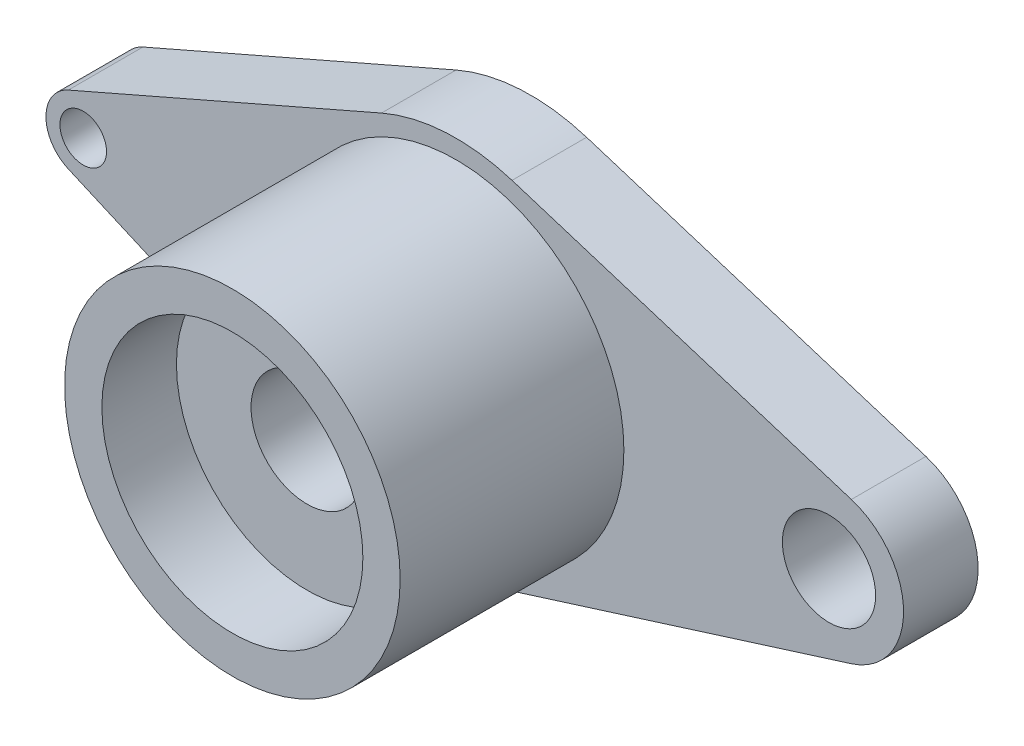
ISO-10303-21;
HEADER;
FILE_DESCRIPTION(('STEP AP214'),'2;1');
FILE_NAME('part.step','',(''),(''),'','','');
FILE_SCHEMA(('AUTOMOTIVE_DESIGN { 1 0 10303 214 1 1 1 1 }'));
ENDSEC;
DATA;
#1=APPLICATION_CONTEXT('core data for automotive mechanical design processes');
#2=APPLICATION_PROTOCOL_DEFINITION('international standard','automotive_design',2000,#1);
#3=PRODUCT_CONTEXT('',#1,'mechanical');
#4=PRODUCT('Part','Part','',(#3));
#5=PRODUCT_RELATED_PRODUCT_CATEGORY('part','',(#4));
#6=PRODUCT_DEFINITION_FORMATION('','',#4);
#7=PRODUCT_DEFINITION_CONTEXT('part definition',#1,'design');
#8=PRODUCT_DEFINITION('design','',#6,#7);
#9=PRODUCT_DEFINITION_SHAPE('','',#8);
#10=(LENGTH_UNIT() NAMED_UNIT(*) SI_UNIT(.MILLI.,.METRE.));
#11=(NAMED_UNIT(*) PLANE_ANGLE_UNIT() SI_UNIT($,.RADIAN.));
#12=(NAMED_UNIT(*) SI_UNIT($,.STERADIAN.) SOLID_ANGLE_UNIT());
#13=UNCERTAINTY_MEASURE_WITH_UNIT(LENGTH_MEASURE(1.E-05),#10,'distance_accuracy_value','');
#14=(GEOMETRIC_REPRESENTATION_CONTEXT(3) GLOBAL_UNCERTAINTY_ASSIGNED_CONTEXT((#13)) GLOBAL_UNIT_ASSIGNED_CONTEXT((#10,
#11,#12)) REPRESENTATION_CONTEXT('',''));
#15=CARTESIAN_POINT('',(0.,0.,0.));
#16=DIRECTION('',(0.,0.,1.));
#17=DIRECTION('',(1.,0.,0.));
#18=AXIS2_PLACEMENT_3D('',#15,#16,#17);
#19=CARTESIAN_POINT('',(0.,0.,20.));
#20=DIRECTION('',(0.,0.,1.));
#21=DIRECTION('',(1.,0.,0.));
#22=AXIS2_PLACEMENT_3D('',#19,#20,#21);
#23=PLANE('',#22);
#24=CARTESIAN_POINT('',(100.,0.,20.));
#25=DIRECTION('',(0.,0.,1.));
#26=DIRECTION('',(1.,0.,0.));
#27=AXIS2_PLACEMENT_3D('',#24,#25,#26);
#28=CIRCLE('',#27,45.);
#29=CARTESIAN_POINT('',(145.,0.,20.));
#30=VERTEX_POINT('',#29);
#31=EDGE_CURVE('E200',#30,#30,#28,.T.);
#32=ORIENTED_EDGE('',*,*,#31,.F.);
#33=EDGE_LOOP('',(#32));
#34=FACE_BOUND('',#33,.T.);
#35=CARTESIAN_POINT('',(0.,0.,20.));
#36=DIRECTION('',(0.,0.,1.));
#37=DIRECTION('',(1.,0.,0.));
#38=AXIS2_PLACEMENT_3D('',#35,#36,#37);
#39=CIRCLE('',#38,6.25);
#40=CARTESIAN_POINT('',(6.25,0.,20.));
#41=VERTEX_POINT('',#40);
#42=EDGE_CURVE('E150',#41,#41,#39,.T.);
#43=ORIENTED_EDGE('',*,*,#42,.F.);
#44=EDGE_LOOP('',(#43));
#45=FACE_BOUND('',#44,.T.);
#46=CARTESIAN_POINT('',(0.,0.,20.));
#47=DIRECTION('',(0.,0.,1.));
#48=DIRECTION('',(1.,0.,0.));
#49=AXIS2_PLACEMENT_3D('',#46,#47,#48);
#50=CIRCLE('',#49,10.);
#51=CARTESIAN_POINT('',(-4.,9.16515138991168,20.));
#52=VERTEX_POINT('',#51);
#53=CARTESIAN_POINT('',(-4.,-9.16515138991168,20.));
#54=VERTEX_POINT('',#53);
#55=EDGE_CURVE('E158',#52,#54,#50,.T.);
#56=ORIENTED_EDGE('',*,*,#55,.T.);
#57=DIRECTION('',(0.916515138991168,-0.4,0.));
#58=VECTOR('',#57,1.);
#59=CARTESIAN_POINT('',(-4.,-9.16515138991168,20.));
#60=LINE('',#59,#58);
#61=CARTESIAN_POINT('',(80.,-45.8257569495584,20.));
#62=VERTEX_POINT('',#61);
#63=EDGE_CURVE('E106',#54,#62,#60,.T.);
#64=ORIENTED_EDGE('',*,*,#63,.T.);
#65=CARTESIAN_POINT('',(100.,0.,20.));
#66=DIRECTION('',(0.,0.,1.));
#67=DIRECTION('',(1.,0.,0.));
#68=AXIS2_PLACEMENT_3D('',#65,#66,#67);
#69=CIRCLE('',#68,50.);
#70=CARTESIAN_POINT('',(115.,-47.6969600708473,20.));
#71=VERTEX_POINT('',#70);
#72=EDGE_CURVE('E212',#62,#71,#69,.T.);
#73=ORIENTED_EDGE('',*,*,#72,.T.);
#74=DIRECTION('',(0.953939201416946,0.3,0.));
#75=VECTOR('',#74,1.);
#76=CARTESIAN_POINT('',(115.,-47.6969600708473,20.));
#77=LINE('',#76,#75);
#78=CARTESIAN_POINT('',(206.,-19.0787840283389,20.));
#79=VERTEX_POINT('',#78);
#80=EDGE_CURVE('E216',#71,#79,#77,.T.);
#81=ORIENTED_EDGE('',*,*,#80,.T.);
#82=CARTESIAN_POINT('',(200.,0.,20.));
#83=DIRECTION('',(0.,0.,1.));
#84=DIRECTION('',(1.,0.,0.));
#85=AXIS2_PLACEMENT_3D('',#82,#83,#84);
#86=CIRCLE('',#85,20.);
#87=CARTESIAN_POINT('',(206.,19.0787840283389,20.));
#88=VERTEX_POINT('',#87);
#89=EDGE_CURVE('E123',#79,#88,#86,.T.);
#90=ORIENTED_EDGE('',*,*,#89,.T.);
#91=DIRECTION('',(-0.953939201416946,0.3,0.));
#92=VECTOR('',#91,1.);
#93=CARTESIAN_POINT('',(115.,47.6969600708473,20.));
#94=LINE('',#93,#92);
#95=CARTESIAN_POINT('',(115.,47.6969600708473,20.));
#96=VERTEX_POINT('',#95);
#97=EDGE_CURVE('E118',#88,#96,#94,.T.);
#98=ORIENTED_EDGE('',*,*,#97,.T.);
#99=CARTESIAN_POINT('',(100.,0.,20.));
#100=DIRECTION('',(0.,0.,1.));
#101=DIRECTION('',(1.,0.,0.));
#102=AXIS2_PLACEMENT_3D('',#99,#100,#101);
#103=CIRCLE('',#102,50.);
#104=CARTESIAN_POINT('',(80.,45.8257569495584,20.));
#105=VERTEX_POINT('',#104);
#106=EDGE_CURVE('E125',#96,#105,#103,.T.);
#107=ORIENTED_EDGE('',*,*,#106,.T.);
#108=DIRECTION('',(-0.916515138991168,-0.4,0.));
#109=VECTOR('',#108,1.);
#110=CARTESIAN_POINT('',(-4.,9.16515138991168,20.));
#111=LINE('',#110,#109);
#112=EDGE_CURVE('E61',#105,#52,#111,.T.);
#113=ORIENTED_EDGE('',*,*,#112,.T.);
#114=EDGE_LOOP('',(#56,#64,#73,#81,#90,#98,#107,#113));
#115=FACE_BOUND('',#114,.T.);
#116=CARTESIAN_POINT('',(200.,0.,20.));
#117=DIRECTION('',(0.,0.,1.));
#118=DIRECTION('',(1.,0.,0.));
#119=AXIS2_PLACEMENT_3D('',#116,#117,#118);
#120=CIRCLE('',#119,12.5);
#121=CARTESIAN_POINT('',(212.5,0.,20.));
#122=VERTEX_POINT('',#121);
#123=EDGE_CURVE('E206',#122,#122,#120,.T.);
#124=ORIENTED_EDGE('',*,*,#123,.F.);
#125=EDGE_LOOP('',(#124));
#126=FACE_BOUND('',#125,.T.);
#127=ADVANCED_FACE('F44',(#34,#45,#115,#126),#23,.T.);
#128=CARTESIAN_POINT('',(0.,0.,0.));
#129=DIRECTION('',(0.,0.,1.));
#130=DIRECTION('',(1.,0.,0.));
#131=AXIS2_PLACEMENT_3D('',#128,#129,#130);
#132=PLANE('',#131);
#133=CARTESIAN_POINT('',(0.,0.,0.));
#134=DIRECTION('',(0.,0.,1.));
#135=DIRECTION('',(1.,0.,0.));
#136=AXIS2_PLACEMENT_3D('',#133,#134,#135);
#137=CIRCLE('',#136,10.);
#138=CARTESIAN_POINT('',(-4.,9.16515138991168,0.));
#139=VERTEX_POINT('',#138);
#140=CARTESIAN_POINT('',(-4.,-9.16515138991168,0.));
#141=VERTEX_POINT('',#140);
#142=EDGE_CURVE('E141',#139,#141,#137,.T.);
#143=ORIENTED_EDGE('',*,*,#142,.F.);
#144=DIRECTION('',(-0.916515138991168,-0.4,0.));
#145=VECTOR('',#144,1.);
#146=CARTESIAN_POINT('',(-4.,9.16515138991168,0.));
#147=LINE('',#146,#145);
#148=CARTESIAN_POINT('',(80.,45.8257569495584,0.));
#149=VERTEX_POINT('',#148);
#150=EDGE_CURVE('E100',#149,#139,#147,.T.);
#151=ORIENTED_EDGE('',*,*,#150,.F.);
#152=CARTESIAN_POINT('',(100.,0.,0.));
#153=DIRECTION('',(0.,0.,1.));
#154=DIRECTION('',(1.,0.,0.));
#155=AXIS2_PLACEMENT_3D('',#152,#153,#154);
#156=CIRCLE('',#155,50.);
#157=CARTESIAN_POINT('',(115.,47.6969600708473,0.));
#158=VERTEX_POINT('',#157);
#159=EDGE_CURVE('E93',#158,#149,#156,.T.);
#160=ORIENTED_EDGE('',*,*,#159,.F.);
#161=DIRECTION('',(-0.953939201416946,0.3,0.));
#162=VECTOR('',#161,1.);
#163=CARTESIAN_POINT('',(115.,47.6969600708473,0.));
#164=LINE('',#163,#162);
#165=CARTESIAN_POINT('',(206.,19.0787840283389,0.));
#166=VERTEX_POINT('',#165);
#167=EDGE_CURVE('E135',#166,#158,#164,.T.);
#168=ORIENTED_EDGE('',*,*,#167,.F.);
#169=CARTESIAN_POINT('',(200.,0.,0.));
#170=DIRECTION('',(0.,0.,1.));
#171=DIRECTION('',(1.,0.,0.));
#172=AXIS2_PLACEMENT_3D('',#169,#170,#171);
#173=CIRCLE('',#172,20.);
#174=CARTESIAN_POINT('',(206.,-19.0787840283389,0.));
#175=VERTEX_POINT('',#174);
#176=EDGE_CURVE('E153',#175,#166,#173,.T.);
#177=ORIENTED_EDGE('',*,*,#176,.F.);
#178=DIRECTION('',(0.953939201416946,0.3,0.));
#179=VECTOR('',#178,1.);
#180=CARTESIAN_POINT('',(115.,-47.6969600708473,0.));
#181=LINE('',#180,#179);
#182=CARTESIAN_POINT('',(115.,-47.6969600708473,0.));
#183=VERTEX_POINT('',#182);
#184=EDGE_CURVE('E151',#183,#175,#181,.T.);
#185=ORIENTED_EDGE('',*,*,#184,.F.);
#186=CARTESIAN_POINT('',(100.,0.,0.));
#187=DIRECTION('',(0.,0.,1.));
#188=DIRECTION('',(1.,0.,0.));
#189=AXIS2_PLACEMENT_3D('',#186,#187,#188);
#190=CIRCLE('',#189,50.);
#191=CARTESIAN_POINT('',(80.,-45.8257569495584,0.));
#192=VERTEX_POINT('',#191);
#193=EDGE_CURVE('E149',#192,#183,#190,.T.);
#194=ORIENTED_EDGE('',*,*,#193,.F.);
#195=DIRECTION('',(0.916515138991168,-0.4,0.));
#196=VECTOR('',#195,1.);
#197=CARTESIAN_POINT('',(-4.,-9.16515138991168,0.));
#198=LINE('',#197,#196);
#199=EDGE_CURVE('E148',#141,#192,#198,.T.);
#200=ORIENTED_EDGE('',*,*,#199,.F.);
#201=EDGE_LOOP('',(#143,#151,#160,#168,#177,#185,#194,#200));
#202=FACE_BOUND('',#201,.T.);
#203=CARTESIAN_POINT('',(0.,0.,0.));
#204=DIRECTION('',(0.,0.,1.));
#205=DIRECTION('',(1.,0.,0.));
#206=AXIS2_PLACEMENT_3D('',#203,#204,#205);
#207=CIRCLE('',#206,6.25);
#208=CARTESIAN_POINT('',(6.25,0.,0.));
#209=VERTEX_POINT('',#208);
#210=EDGE_CURVE('E201',#209,#209,#207,.T.);
#211=ORIENTED_EDGE('',*,*,#210,.T.);
#212=EDGE_LOOP('',(#211));
#213=FACE_BOUND('',#212,.T.);
#214=CARTESIAN_POINT('',(200.,0.,0.));
#215=DIRECTION('',(0.,0.,1.));
#216=DIRECTION('',(1.,0.,0.));
#217=AXIS2_PLACEMENT_3D('',#214,#215,#216);
#218=CIRCLE('',#217,12.5);
#219=CARTESIAN_POINT('',(212.5,0.,0.));
#220=VERTEX_POINT('',#219);
#221=EDGE_CURVE('E207',#220,#220,#218,.T.);
#222=ORIENTED_EDGE('',*,*,#221,.T.);
#223=EDGE_LOOP('',(#222));
#224=FACE_BOUND('',#223,.T.);
#225=ADVANCED_FACE('F188',(#202,#213,#224),#132,.F.);
#226=CARTESIAN_POINT('',(0.,0.,20.));
#227=DIRECTION('',(0.,0.,-1.));
#228=DIRECTION('',(-1.,0.,0.));
#229=AXIS2_PLACEMENT_3D('',#226,#227,#228);
#230=CYLINDRICAL_SURFACE('',#229,10.);
#231=ORIENTED_EDGE('',*,*,#142,.T.);
#232=DIRECTION('',(0.,0.,-1.));
#233=VECTOR('',#232,1.);
#234=CARTESIAN_POINT('',(-4.,-9.16515138991168,20.));
#235=LINE('',#234,#233);
#236=EDGE_CURVE('E174',#54,#141,#235,.T.);
#237=ORIENTED_EDGE('',*,*,#236,.F.);
#238=ORIENTED_EDGE('',*,*,#55,.F.);
#239=DIRECTION('',(0.,0.,-1.));
#240=VECTOR('',#239,1.);
#241=CARTESIAN_POINT('',(-4.,9.16515138991168,20.));
#242=LINE('',#241,#240);
#243=EDGE_CURVE('E136',#52,#139,#242,.T.);
#244=ORIENTED_EDGE('',*,*,#243,.T.);
#245=EDGE_LOOP('',(#231,#237,#238,#244));
#246=FACE_BOUND('',#245,.T.);
#247=ADVANCED_FACE('F50',(#246),#230,.T.);
#248=CARTESIAN_POINT('',(-4.,-9.16515138991168,20.));
#249=DIRECTION('',(0.4,0.916515138991168,0.));
#250=DIRECTION('',(-0.916515138991168,0.4,0.));
#251=AXIS2_PLACEMENT_3D('',#248,#249,#250);
#252=PLANE('',#251);
#253=ORIENTED_EDGE('',*,*,#199,.T.);
#254=DIRECTION('',(0.,0.,-1.));
#255=VECTOR('',#254,1.);
#256=CARTESIAN_POINT('',(80.,-45.8257569495584,20.));
#257=LINE('',#256,#255);
#258=EDGE_CURVE('E169',#62,#192,#257,.T.);
#259=ORIENTED_EDGE('',*,*,#258,.F.);
#260=ORIENTED_EDGE('',*,*,#63,.F.);
#261=ORIENTED_EDGE('',*,*,#236,.T.);
#262=EDGE_LOOP('',(#253,#259,#260,#261));
#263=FACE_BOUND('',#262,.T.);
#264=ADVANCED_FACE('F251',(#263),#252,.F.);
#265=CARTESIAN_POINT('',(100.,0.,20.));
#266=DIRECTION('',(0.,0.,-1.));
#267=DIRECTION('',(-1.,0.,0.));
#268=AXIS2_PLACEMENT_3D('',#265,#266,#267);
#269=CYLINDRICAL_SURFACE('',#268,50.);
#270=ORIENTED_EDGE('',*,*,#193,.T.);
#271=DIRECTION('',(0.,0.,-1.));
#272=VECTOR('',#271,1.);
#273=CARTESIAN_POINT('',(115.,-47.6969600708473,20.));
#274=LINE('',#273,#272);
#275=EDGE_CURVE('E164',#71,#183,#274,.T.);
#276=ORIENTED_EDGE('',*,*,#275,.F.);
#277=ORIENTED_EDGE('',*,*,#72,.F.);
#278=ORIENTED_EDGE('',*,*,#258,.T.);
#279=EDGE_LOOP('',(#270,#276,#277,#278));
#280=FACE_BOUND('',#279,.T.);
#281=ADVANCED_FACE('F253',(#280),#269,.T.);
#282=CARTESIAN_POINT('',(115.,-47.6969600708473,20.));
#283=DIRECTION('',(-0.3,0.953939201416946,0.));
#284=DIRECTION('',(-0.953939201416946,-0.3,0.));
#285=AXIS2_PLACEMENT_3D('',#282,#283,#284);
#286=PLANE('',#285);
#287=ORIENTED_EDGE('',*,*,#184,.T.);
#288=DIRECTION('',(0.,0.,-1.));
#289=VECTOR('',#288,1.);
#290=CARTESIAN_POINT('',(206.,-19.0787840283389,20.));
#291=LINE('',#290,#289);
#292=EDGE_CURVE('E165',#79,#175,#291,.T.);
#293=ORIENTED_EDGE('',*,*,#292,.F.);
#294=ORIENTED_EDGE('',*,*,#80,.F.);
#295=ORIENTED_EDGE('',*,*,#275,.T.);
#296=EDGE_LOOP('',(#287,#293,#294,#295));
#297=FACE_BOUND('',#296,.T.);
#298=ADVANCED_FACE('F225',(#297),#286,.F.);
#299=CARTESIAN_POINT('',(200.,0.,20.));
#300=DIRECTION('',(0.,0.,-1.));
#301=DIRECTION('',(-1.,0.,0.));
#302=AXIS2_PLACEMENT_3D('',#299,#300,#301);
#303=CYLINDRICAL_SURFACE('',#302,20.);
#304=ORIENTED_EDGE('',*,*,#176,.T.);
#305=DIRECTION('',(0.,0.,-1.));
#306=VECTOR('',#305,1.);
#307=CARTESIAN_POINT('',(206.,19.0787840283389,20.));
#308=LINE('',#307,#306);
#309=EDGE_CURVE('E133',#88,#166,#308,.T.);
#310=ORIENTED_EDGE('',*,*,#309,.F.);
#311=ORIENTED_EDGE('',*,*,#89,.F.);
#312=ORIENTED_EDGE('',*,*,#292,.T.);
#313=EDGE_LOOP('',(#304,#310,#311,#312));
#314=FACE_BOUND('',#313,.T.);
#315=ADVANCED_FACE('F229',(#314),#303,.T.);
#316=CARTESIAN_POINT('',(115.,47.6969600708473,20.));
#317=DIRECTION('',(-0.3,-0.953939201416946,0.));
#318=DIRECTION('',(0.953939201416946,-0.3,0.));
#319=AXIS2_PLACEMENT_3D('',#316,#317,#318);
#320=PLANE('',#319);
#321=ORIENTED_EDGE('',*,*,#167,.T.);
#322=DIRECTION('',(0.,0.,-1.));
#323=VECTOR('',#322,1.);
#324=CARTESIAN_POINT('',(115.,47.6969600708473,20.));
#325=LINE('',#324,#323);
#326=EDGE_CURVE('E128',#96,#158,#325,.T.);
#327=ORIENTED_EDGE('',*,*,#326,.F.);
#328=ORIENTED_EDGE('',*,*,#97,.F.);
#329=ORIENTED_EDGE('',*,*,#309,.T.);
#330=EDGE_LOOP('',(#321,#327,#328,#329));
#331=FACE_BOUND('',#330,.T.);
#332=ADVANCED_FACE('F134',(#331),#320,.F.);
#333=CARTESIAN_POINT('',(100.,0.,20.));
#334=DIRECTION('',(0.,0.,-1.));
#335=DIRECTION('',(-1.,0.,0.));
#336=AXIS2_PLACEMENT_3D('',#333,#334,#335);
#337=CYLINDRICAL_SURFACE('',#336,50.);
#338=ORIENTED_EDGE('',*,*,#159,.T.);
#339=DIRECTION('',(0.,0.,-1.));
#340=VECTOR('',#339,1.);
#341=CARTESIAN_POINT('',(80.,45.8257569495584,20.));
#342=LINE('',#341,#340);
#343=EDGE_CURVE('E132',#105,#149,#342,.T.);
#344=ORIENTED_EDGE('',*,*,#343,.F.);
#345=ORIENTED_EDGE('',*,*,#106,.F.);
#346=ORIENTED_EDGE('',*,*,#326,.T.);
#347=EDGE_LOOP('',(#338,#344,#345,#346));
#348=FACE_BOUND('',#347,.T.);
#349=ADVANCED_FACE('F139',(#348),#337,.T.);
#350=CARTESIAN_POINT('',(-4.,9.16515138991168,20.));
#351=DIRECTION('',(0.4,-0.916515138991168,0.));
#352=DIRECTION('',(0.916515138991168,0.4,0.));
#353=AXIS2_PLACEMENT_3D('',#350,#351,#352);
#354=PLANE('',#353);
#355=ORIENTED_EDGE('',*,*,#150,.T.);
#356=ORIENTED_EDGE('',*,*,#243,.F.);
#357=ORIENTED_EDGE('',*,*,#112,.F.);
#358=ORIENTED_EDGE('',*,*,#343,.T.);
#359=EDGE_LOOP('',(#355,#356,#357,#358));
#360=FACE_BOUND('',#359,.T.);
#361=ADVANCED_FACE('F235',(#360),#354,.F.);
#362=CARTESIAN_POINT('',(0.,0.,20.));
#363=DIRECTION('',(0.,0.,-1.));
#364=DIRECTION('',(-1.,0.,0.));
#365=AXIS2_PLACEMENT_3D('',#362,#363,#364);
#366=CYLINDRICAL_SURFACE('',#365,6.25);
#367=ORIENTED_EDGE('',*,*,#42,.T.);
#368=EDGE_LOOP('',(#367));
#369=FACE_BOUND('',#368,.T.);
#370=ORIENTED_EDGE('',*,*,#210,.F.);
#371=EDGE_LOOP('',(#370));
#372=FACE_BOUND('',#371,.T.);
#373=ADVANCED_FACE('F233',(#369,#372),#366,.F.);
#374=CARTESIAN_POINT('',(200.,0.,20.));
#375=DIRECTION('',(0.,0.,-1.));
#376=DIRECTION('',(-1.,0.,0.));
#377=AXIS2_PLACEMENT_3D('',#374,#375,#376);
#378=CYLINDRICAL_SURFACE('',#377,12.5);
#379=ORIENTED_EDGE('',*,*,#123,.T.);
#380=EDGE_LOOP('',(#379));
#381=FACE_BOUND('',#380,.T.);
#382=ORIENTED_EDGE('',*,*,#221,.F.);
#383=EDGE_LOOP('',(#382));
#384=FACE_BOUND('',#383,.T.);
#385=ADVANCED_FACE('F241',(#381,#384),#378,.F.);
#386=CARTESIAN_POINT('',(100.,0.,80.));
#387=DIRECTION('',(0.,0.,1.));
#388=DIRECTION('',(1.,0.,0.));
#389=AXIS2_PLACEMENT_3D('',#386,#387,#388);
#390=PLANE('',#389);
#391=CARTESIAN_POINT('',(100.,0.,80.));
#392=DIRECTION('',(0.,0.,1.));
#393=DIRECTION('',(1.,0.,0.));
#394=AXIS2_PLACEMENT_3D('',#391,#392,#393);
#395=CIRCLE('',#394,45.);
#396=CARTESIAN_POINT('',(145.,0.,80.));
#397=VERTEX_POINT('',#396);
#398=EDGE_CURVE('E462',#397,#397,#395,.T.);
#399=ORIENTED_EDGE('',*,*,#398,.T.);
#400=EDGE_LOOP('',(#399));
#401=FACE_BOUND('',#400,.T.);
#402=CARTESIAN_POINT('',(100.,0.,80.));
#403=DIRECTION('',(0.,0.,1.));
#404=DIRECTION('',(1.,0.,0.));
#405=AXIS2_PLACEMENT_3D('',#402,#403,#404);
#406=CIRCLE('',#405,35.);
#407=CARTESIAN_POINT('',(135.,0.,80.));
#408=VERTEX_POINT('',#407);
#409=EDGE_CURVE('E466',#408,#408,#406,.T.);
#410=ORIENTED_EDGE('',*,*,#409,.F.);
#411=EDGE_LOOP('',(#410));
#412=FACE_BOUND('',#411,.T.);
#413=ADVANCED_FACE('F308',(#401,#412),#390,.T.);
#414=CARTESIAN_POINT('',(100.,0.,80.));
#415=DIRECTION('',(0.,0.,-1.));
#416=DIRECTION('',(-1.,0.,0.));
#417=AXIS2_PLACEMENT_3D('',#414,#415,#416);
#418=CYLINDRICAL_SURFACE('',#417,45.);
#419=ORIENTED_EDGE('',*,*,#398,.F.);
#420=EDGE_LOOP('',(#419));
#421=FACE_BOUND('',#420,.T.);
#422=ORIENTED_EDGE('',*,*,#31,.T.);
#423=EDGE_LOOP('',(#422));
#424=FACE_BOUND('',#423,.T.);
#425=ADVANCED_FACE('F310',(#421,#424),#418,.T.);
#426=CARTESIAN_POINT('',(100.,0.,80.));
#427=DIRECTION('',(0.,0.,-1.));
#428=DIRECTION('',(-1.,0.,0.));
#429=AXIS2_PLACEMENT_3D('',#426,#427,#428);
#430=CYLINDRICAL_SURFACE('',#429,35.);
#431=CARTESIAN_POINT('',(100.,0.,60.));
#432=DIRECTION('',(0.,0.,1.));
#433=DIRECTION('',(1.,0.,0.));
#434=AXIS2_PLACEMENT_3D('',#431,#432,#433);
#435=CIRCLE('',#434,35.);
#436=CARTESIAN_POINT('',(135.,0.,60.));
#437=VERTEX_POINT('',#436);
#438=EDGE_CURVE('E11',#437,#437,#435,.T.);
#439=ORIENTED_EDGE('',*,*,#438,.F.);
#440=EDGE_LOOP('',(#439));
#441=FACE_BOUND('',#440,.T.);
#442=ORIENTED_EDGE('',*,*,#409,.T.);
#443=EDGE_LOOP('',(#442));
#444=FACE_BOUND('',#443,.T.);
#445=ADVANCED_FACE('F317',(#441,#444),#430,.F.);
#446=CARTESIAN_POINT('',(100.,0.,60.));
#447=DIRECTION('',(0.,0.,1.));
#448=DIRECTION('',(1.,0.,0.));
#449=AXIS2_PLACEMENT_3D('',#446,#447,#448);
#450=PLANE('',#449);
#451=ORIENTED_EDGE('',*,*,#438,.T.);
#452=EDGE_LOOP('',(#451));
#453=FACE_BOUND('',#452,.T.);
#454=CARTESIAN_POINT('',(100.,0.,60.));
#455=DIRECTION('',(0.,0.,1.));
#456=DIRECTION('',(1.,0.,0.));
#457=AXIS2_PLACEMENT_3D('',#454,#455,#456);
#458=CIRCLE('',#457,15.);
#459=CARTESIAN_POINT('',(115.,0.,60.));
#460=VERTEX_POINT('',#459);
#461=EDGE_CURVE('E475',#460,#460,#458,.T.);
#462=ORIENTED_EDGE('',*,*,#461,.F.);
#463=EDGE_LOOP('',(#462));
#464=FACE_BOUND('',#463,.T.);
#465=ADVANCED_FACE('F181',(#453,#464),#450,.T.);
#466=CARTESIAN_POINT('',(100.,0.,60.));
#467=DIRECTION('',(0.,0.,-1.));
#468=DIRECTION('',(-1.,0.,0.));
#469=AXIS2_PLACEMENT_3D('',#466,#467,#468);
#470=CYLINDRICAL_SURFACE('',#469,15.);
#471=ORIENTED_EDGE('',*,*,#461,.T.);
#472=EDGE_LOOP('',(#471));
#473=FACE_BOUND('',#472,.T.);
#474=CARTESIAN_POINT('',(100.,0.,20.));
#475=DIRECTION('',(0.,0.,1.));
#476=DIRECTION('',(1.,0.,0.));
#477=AXIS2_PLACEMENT_3D('',#474,#475,#476);
#478=CIRCLE('',#477,15.);
#479=CARTESIAN_POINT('',(115.,0.,20.));
#480=VERTEX_POINT('',#479);
#481=EDGE_CURVE('E53',#480,#480,#478,.F.);
#482=ORIENTED_EDGE('',*,*,#481,.T.);
#483=EDGE_LOOP('',(#482));
#484=FACE_BOUND('',#483,.T.);
#485=ADVANCED_FACE('F172',(#473,#484),#470,.F.);
#486=ORIENTED_EDGE('',*,*,#481,.F.);
#487=EDGE_LOOP('',(#486));
#488=FACE_BOUND('',#487,.T.);
#489=ADVANCED_FACE('F179',(#488),#23,.T.);
#490=CLOSED_SHELL('',(#127,#225,#247,#264,#281,#298,#315,#332,#349,#361,#373,#385,#413,#425,
#445,#465,#485,#489));
#491=MANIFOLD_SOLID_BREP('B2',#490);
#492=ADVANCED_BREP_SHAPE_REPRESENTATION('',(#18,#491),#14);
#493=SHAPE_DEFINITION_REPRESENTATION(#9,#492);
ENDSEC;
END-ISO-10303-21;
